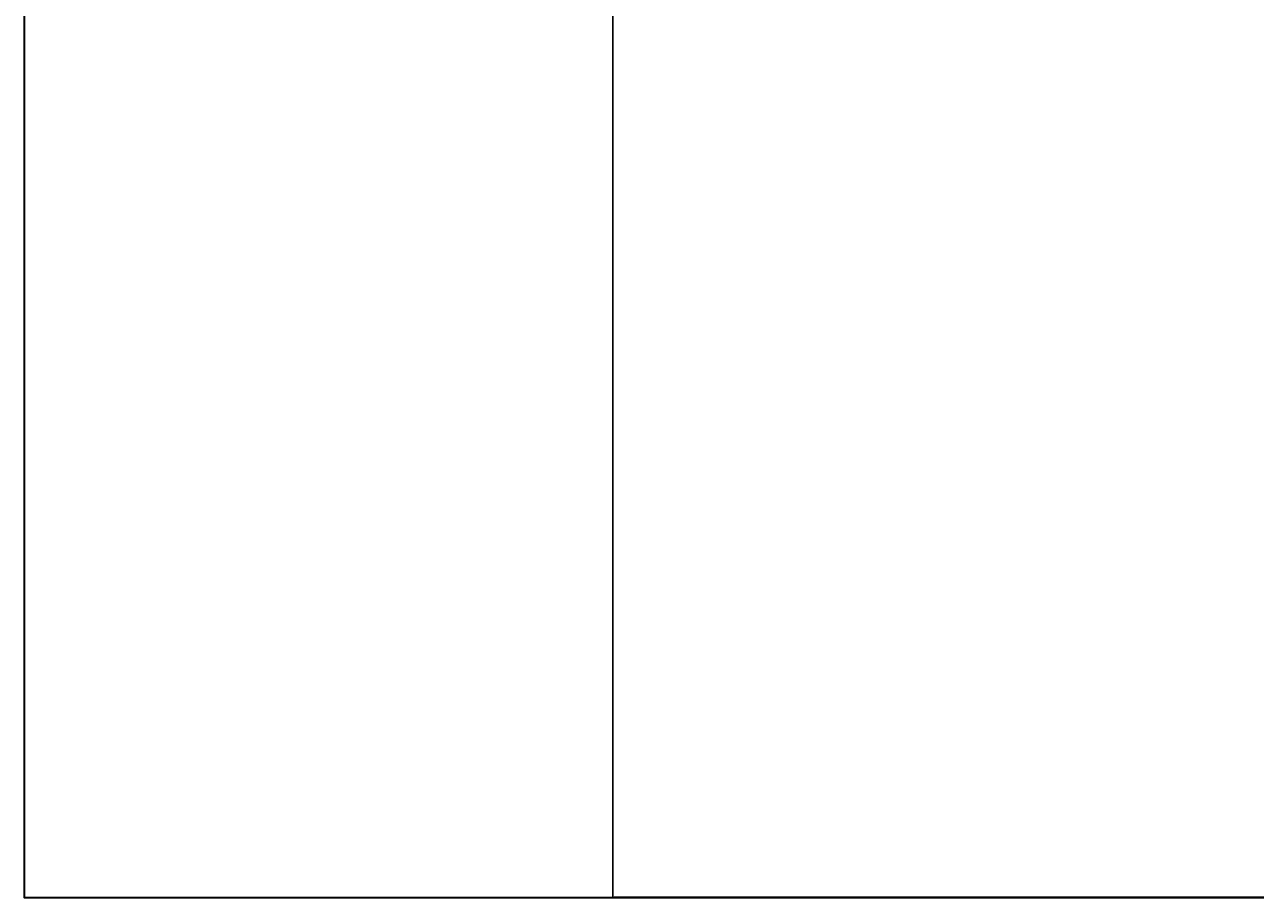
# Model space of a CAD drawing. Units: inches. Extents: x 1885 to 2748, y 783 to 2421.
# Tile 1 of 117: x 1885 to 2065, y 922 to 1050. Entities that reach past the tile are written whole.
import ezdxf

# ---------------------------------------------------------------- set-up
doc = ezdxf.new("R2010")
doc.units = ezdxf.units.IN
doc.layers.add('A-ANNO-DIMS', color=2, linetype='Continuous', lineweight=18)
doc.layers.add('A-ANNO-TTLB', color=7, linetype='Continuous', lineweight=35)
doc.styles.get("Standard").update_dxf_attribs({"font": 'arial.ttf'})
doc.dimstyles.get("Standard").update_dxf_attribs({"dimtxt": 0.18, "dimasz": 0.18, "dimexe": 0.18, "dimexo": 0.0625, "dimgap": 0.09, "dimtad": 0, "dimtih": 1, "dimtoh": 1, "dimdec": 4, "dimzin": 0, "dimdsep": 46, "dimtxsty": 'Standard', "dimcen": 0.09, "dimadec": 0, "dimazin": 0, "dimtfac": 1, "dimtdec": 4, "dimtofl": 0, "dimtmove": 0, "dimatfit": 3, "dimfxl": 1, "dimtolj": 1, "dimtzin": 0, "dimarcsym": 0})

# ---------------------------------------------------------------- blocks, each defined once
blk = doc.blocks.new('*D43')
at = {"layer": 'A-ANNO-DIMS', "color": 0, "lineweight": -2, "transparency": 16777216}
for p, q in [((1971.27, 1057.44), (1971.27, 922.48)), ((2618.27, 1057.44), (2618.27, 922.48)), ((1971.45, 922.66), (2294.48, 922.66)), ((2618.09, 922.66), (2295.06, 922.66))]:
    blk.add_line(p, q, dxfattribs=at)
at = {"layer": 'A-ANNO-DIMS', "color": 0, "transparency": 16777216}
for points in [[(1971.45, 922.69), (1971.45, 922.63), (1971.27, 922.66)], [(2618.09, 922.69), (2618.09, 922.63), (2618.27, 922.66)]]:
    blk.add_solid(points, dxfattribs=at)
at = {"layer": 'Defpoints', "color": 0, "transparency": 16777216}
for p in [(1971.27, 1057.51), (2618.27, 1057.51), (2618.27, 922.66)]:
    blk.add_point(p, dxfattribs=at)
at = {"layer": 'A-ANNO-DIMS', "color": 0, "transparency": 16777216, "insert": (2294.77, 922.66), "char_height": 0.18, "attachment_point": 5}
blk.add_mtext('\\A1;647', dxfattribs=at)

msp = doc.modelspace()

# ---------------------------------------------------------------- linework, layer by layer
at = {"layer": 'A-ANNO-TTLB'}
msp.add_lwpolyline([(1885.16, 2409.17), (2748.2, 2409.17), (2748.2, 922.58), (1885.16, 922.58)], close=True, dxfattribs=at)

# ---------------------------------------------------------------- dimensions: what is measured, and where the dimension line sits
at = {"layer": 'A-ANNO-DIMS'}
dim = msp.add_linear_dim(base=(2618.27, 922.66), p1=(1971.27, 1057.51), p2=(2618.27, 1057.51), dimstyle='Standard', override={"dimdec": 0, "dimlfac": 1, "dimrnd": 0, "dimzin": 0, "dimdsep": 46, "dimlunit": 2}, dxfattribs=at)
dim.commit()
dim.dimension.update_dxf_attribs({"geometry": '*D43', "text_midpoint": (2294.77, 922.66)})

doc.saveas('drawing.dxf')
